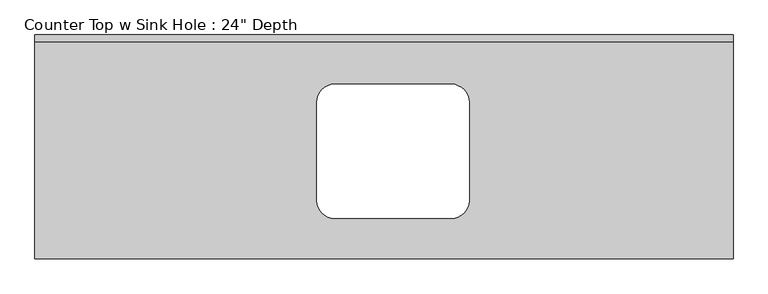
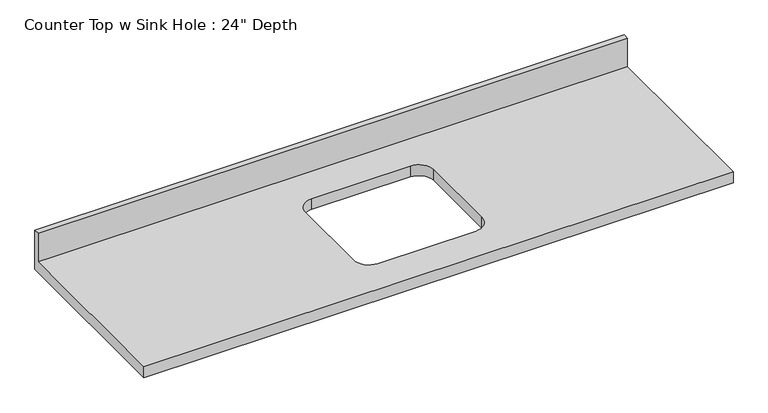
"""IFC4 building model written with IfcOpenShell, lengths in millimetres: furniture geometry."""

from ifc_helpers import new_model, si_unit, frame, origin, place, context, project, spatial, polyline, circle_curve, source, transform, mapped, element, save
from ifc_brep_helpers import plane_surface, revolved_surface, advanced_brep


def furniture_c6510c7c(model_context):
    return source(origin(), model_context, "Body", "AdvancedBrep", [
        advanced_brep(
        [(-1200.4622951, -635.0, 914.4), (780.7377049, -635.0, 914.4), (780.7377049, -19.05, 914.4), (-1200.4622951, -19.05, 914.4), (-349.5622951, -139.7, 914.4), (-19.3622951, -139.7, 914.4), (31.4377049, -190.5, 914.4), (31.4377049, -469.9, 914.4), (-19.3622951, -520.7, 914.4), (-349.5622951, -520.7, 914.4), (-400.3622951, -469.9, 914.4), (-400.3622951, -190.5, 914.4), (780.7377049, 0.0, 876.3), (780.7377049, -635.0, 876.3), (-1200.4622951, -635.0, 876.3), (-1200.4622951, 0.0, 876.3), (-19.3622951, -139.7, 876.3), (-349.5622951, -139.7, 876.3), (-400.3622951, -190.5, 876.3), (-400.3622951, -469.9, 876.3), (-349.5622951, -520.7, 876.3), (-19.3622951, -520.7, 876.3), (31.4377049, -469.9, 876.3), (31.4377049, -190.5, 876.3), (-1200.4622951, 0.0, 1016.0), (780.7377049, 0.0, 1016.0), (-1200.4622951, -19.05, 1016.0), (780.7377049, -19.05, 1016.0)],
        [
            (0, 1),
            (1, 2),
            (2, 3),
            (3, 0),
            (4, 5),
            (5, 6, circle_curve(frame((-19.3622951, -190.5, 914.4), z_axis=(0.0, 0.0, -1.0), x_axis=(1.0, 0.0, 0.0)), 50.8)),
            (6, 7),
            (7, 8, circle_curve(frame((-19.3622951, -469.9, 914.4), z_axis=(0.0, 0.0, -1.0), x_axis=(1.0, 0.0, 0.0)), 50.8)),
            (8, 9),
            (9, 10, circle_curve(frame((-349.5622951, -469.9, 914.4), z_axis=(0.0, 0.0, -1.0), x_axis=(1.0, 0.0, 0.0)), 50.8)),
            (10, 11),
            (11, 4, circle_curve(frame((-349.5622951, -190.5, 914.4), z_axis=(0.0, 0.0, -1.0), x_axis=(1.0, 0.0, 0.0)), 50.8)),
            (12, 13),
            (13, 14),
            (14, 15),
            (15, 12),
            (16, 17),
            (17, 18, circle_curve(frame((-349.5622951, -190.5, 876.3), z_axis=(0.0, 0.0, 1.0), x_axis=(1.0, 0.0, 0.0)), 50.8)),
            (18, 19),
            (19, 20, circle_curve(frame((-349.5622951, -469.9, 876.3), z_axis=(0.0, 0.0, 1.0), x_axis=(1.0, 0.0, 0.0)), 50.8)),
            (20, 21),
            (21, 22, circle_curve(frame((-19.3622951, -469.9, 876.3), z_axis=(0.0, 0.0, 1.0), x_axis=(1.0, 0.0, 0.0)), 50.8)),
            (22, 23),
            (23, 16, circle_curve(frame((-19.3622951, -190.5, 876.3), z_axis=(0.0, 0.0, 1.0), x_axis=(1.0, 0.0, 0.0)), 50.8)),
            (15, 24),
            (24, 25),
            (25, 12),
            (14, 0),
            (3, 26),
            (26, 24),
            (13, 1),
            (25, 27),
            (27, 2),
            (4, 17),
            (16, 5),
            (11, 18),
            (10, 19),
            (9, 20),
            (8, 21),
            (7, 22),
            (6, 23),
            (26, 27),
        ],
        [
            plane_surface(frame((-1200.4622951, 0.0, 914.4), z_axis=(0.0, 0.0, 1.0), x_axis=(-1.0, 0.0, 0.0))),
            plane_surface(frame((-1200.4622951, 0.0, 876.3), z_axis=(0.0, 0.0, -1.0), x_axis=(1.0, 0.0, 0.0))),
            plane_surface(frame((780.7377049, 0.0, 914.4), z_axis=(0.0, 1.0, 0.0), x_axis=(0.0, 0.0, -1.0))),
            plane_surface(frame((-1200.4622951, 0.0, 914.4), z_axis=(-1.0, 0.0, 0.0), x_axis=(0.0, 0.0, -1.0))),
            plane_surface(frame((-1200.4622951, -635.0, 914.4), z_axis=(0.0, -1.0, 0.0), x_axis=(0.0, 0.0, -1.0))),
            plane_surface(frame((780.7377049, -635.0, 914.4), z_axis=(1.0, 0.0, 0.0), x_axis=(0.0, 0.0, -1.0))),
            plane_surface(frame((-19.3622951, -139.7, 914.4), z_axis=(0.0, -1.0, 0.0), x_axis=(0.0, 0.0, -1.0))),
            revolved_surface(polyline([(-298.76229509999996, -190.5, 914.4), (-298.76229509999996, -190.5, 876.3)]), (-349.5622951, -190.5, 876.3), (0.0, 0.0, 1.0)),
            plane_surface(frame((-400.3622951, -190.5, 914.4), z_axis=(1.0, 0.0, 0.0), x_axis=(0.0, 0.0, -1.0))),
            revolved_surface(polyline([(-298.76229509999996, -469.9, 914.4), (-298.76229509999996, -469.9, 876.3)]), (-349.5622951, -469.9, 876.3), (0.0, 0.0, 1.0)),
            plane_surface(frame((-349.5622951, -520.7, 914.4), z_axis=(0.0, 1.0, 0.0), x_axis=(0.0, 0.0, -1.0))),
            revolved_surface(polyline([(31.437704899999996, -469.9, 914.4), (31.437704899999996, -469.9, 876.3)]), (-19.3622951, -469.9, 876.3), (0.0, 0.0, 1.0)),
            plane_surface(frame((31.4377049, -469.9, 914.4), z_axis=(-1.0, 0.0, 0.0), x_axis=(0.0, 0.0, -1.0))),
            revolved_surface(polyline([(31.437704899999996, -190.5, 914.4), (31.437704899999996, -190.5, 876.3)]), (-19.3622951, -190.5, 876.3), (0.0, 0.0, 1.0)),
            plane_surface(frame((-1200.4622951, 0.0, 1016.0), z_axis=(0.0, 0.0, 1.0), x_axis=(0.0, -1.0, 0.0))),
            plane_surface(frame((-1200.4622951, -19.05, 1016.0), z_axis=(0.0, -1.0, 0.0), x_axis=(0.0, 0.0, -1.0))),
        ],
        [
            (0, [[1, 2, 3, 4], [5, 6, 7, 8, 9, 10, 11, 12]]),
            (1, [[13, 14, 15, 16], [17, 18, 19, 20, 21, 22, 23, 24]]),
            (2, [[-16, 25, 26, 27]]),
            (3, [[-15, 28, -4, 29, 30, -25]]),
            (4, [[-1, -28, -14, 31]]),
            (5, [[-13, -27, 32, 33, -2, -31]]),
            (6, [[34, -17, 35, -5]]),
            (7, [[-34, -12, 36, -18]]),
            (8, [[-36, -11, 37, -19]]),
            (9, [[-37, -10, 38, -20]]),
            (10, [[-38, -9, 39, -21]]),
            (11, [[-39, -8, 40, -22]]),
            (12, [[-40, -7, 41, -23]]),
            (13, [[-35, -24, -41, -6]]),
            (14, [[-30, 42, -32, -26]]),
            (15, [[-42, -29, -3, -33]]),
        ],
    ),
    ])


if __name__ == "__main__":
    model = new_model("IFC4")
    model_context = context("Model", 3, world=origin())
    ifc_project = project(units=[si_unit("LENGTHUNIT", "METRE", prefix="MILLI")], contexts=[model_context])
    site = spatial("IfcSite", under=ifc_project)
    building = spatial("IfcBuilding", under=site)
    placement = place(None, origin())
    furniture_shape = furniture_c6510c7c(model_context)
    element("IfcFurniture", 1, ObjectType="Counter Top w Sink Hole : 24\" Depth", at=placement, inside=building, context=model_context, shape_type="MappedRepresentation", body=[
        mapped(furniture_shape, transform((0.0, 0.0, 0.0), x_axis=(1.0, 0.0, 0.0), y_axis=(0.0, 1.0, 0.0), z_axis=(0.0, 0.0, 1.0))),
    ])
    save(model, "model.ifc")

# Revit data of these elements
# Type "Counter Top w Sink Hole : 24\" Depth"
#   Assembly Code = "C1030400"
#   Counter Thickness = 0' - 1 1/2"
#   Depth [instance default] = 2' - 1"
#   Height = 3' - 0"
#   Length [instance default] = 8' - 0"
#   Sink Location [instance default] = 2' - 0"
#   Sink Location To Wall [instance default] = 0' - 6"
#   Sink Opening Depth [instance default] = 1' - 3"
#   Sink Opening Width [instance default] = 2' - 3"
#   Counter Top Material = none
#   Default Elevation = 0
# Element 1 (IfcFurniture, "Counter Top w Sink Hole : 24\" Depth")
#   Length = 6' - 6"
#   Sink Location = 3' - 4"
#   Sink Opening Depth = 1' - 2"
#   Sink Opening Width = 1' - 4"
#   Materials on its faces: "Counter Top"
# Materials
#   "Counter Top": class "Wood", colour RGB 226 177 128, transparency 0
